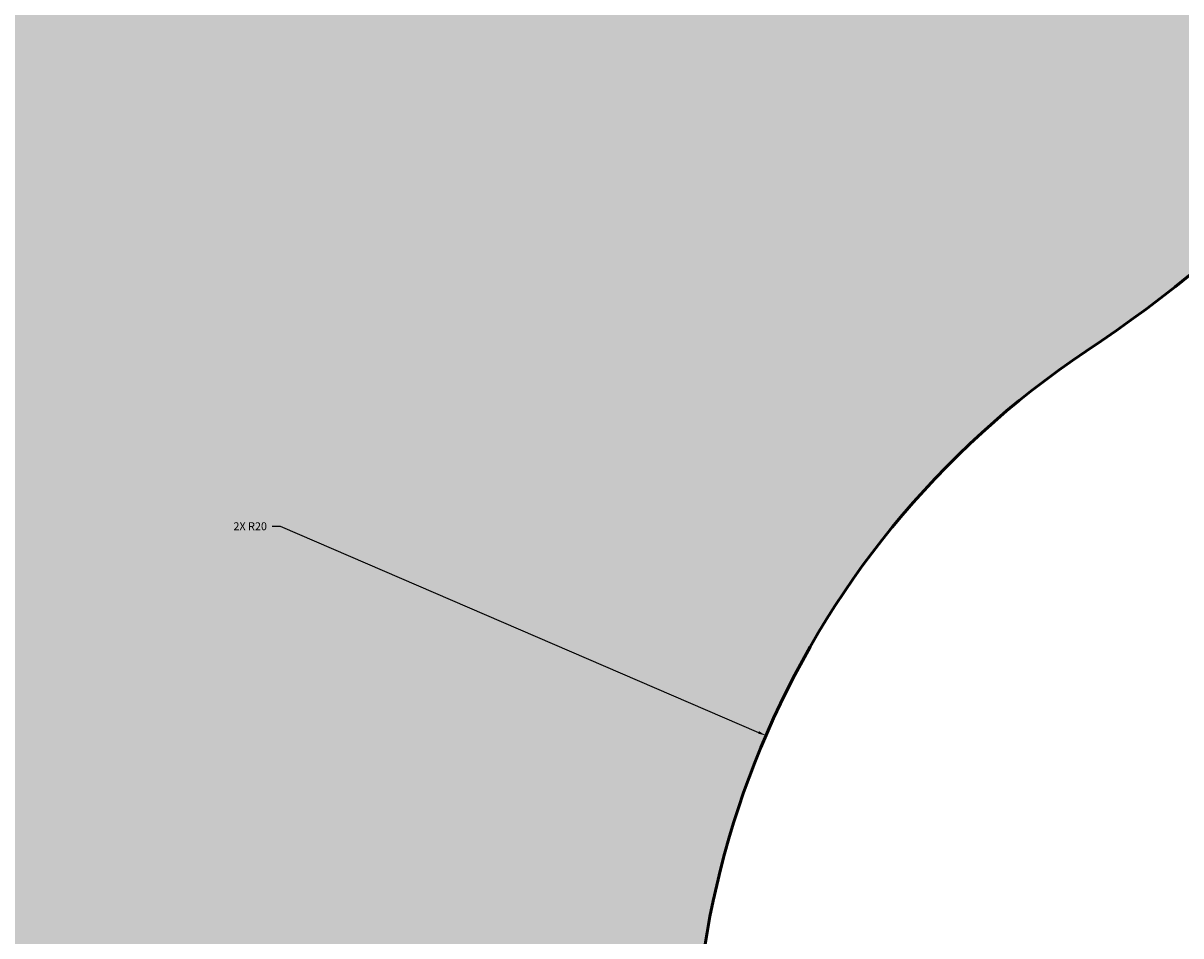
# Model space of a CAD drawing. Units: inches. Extents: x -13 to 107, y -48 to 102.
# Tile 3 of 13: x 22 to 48, y -27 to -7. Entities that reach past the tile are written whole.
import ezdxf

# ---------------------------------------------------------------- set-up
doc = ezdxf.new("R2010")
doc.units = ezdxf.units.IN
doc.header["$MEASUREMENT"] = 0
for name, color, linetype, lineweight in [('M-DIMS', 2, 'Continuous', 18), ('M-HATC', 8, 'Continuous', 18), ('M-OUTL', 7, 'Continuous', 50)]:
    doc.layers.add(name, color=color, linetype=linetype, lineweight=lineweight)
doc.styles.get("Standard").update_dxf_attribs({"font": 'arial.ttf'})
doc.dimstyles.get("Standard").update_dxf_attribs({"dimtxt": 0.18, "dimasz": 0.18, "dimexe": 0.18, "dimexo": 0.0625, "dimgap": 0.09, "dimtad": 0, "dimtih": 1, "dimtoh": 1, "dimdec": 4, "dimzin": 0, "dimdsep": 46, "dimtxsty": 'Standard', "dimcen": 0.09, "dimadec": 0, "dimazin": 0, "dimtfac": 1, "dimtdec": 4, "dimtofl": 0, "dimtmove": 0, "dimatfit": 3, "dimfxl": 1, "dimtolj": 1, "dimtzin": 0, "dimarcsym": 0})

# ---------------------------------------------------------------- blocks, each defined once
blk = doc.blocks.new('*D2')
at = {"layer": 'Defpoints', "color": 0, "transparency": 16777216}
for p in [(-12.585, 94.408), (27.547, 94.408), (27.547, -46.592)]:
    blk.add_point(p, dxfattribs=at)
at = {"layer": 'M-DIMS', "color": 0, "lineweight": -2, "transparency": 16777216}
for p, q in [((27.484, 94.408), (-12.765, 94.408)), ((-12.585, 94.228), (-12.585, 24.088)), ((-12.585, -46.412), (-12.585, 23.727)), ((27.484, -46.592), (-12.765, -46.592))]:
    blk.add_line(p, q, dxfattribs=at)
at = {"layer": 'M-DIMS', "color": 0, "transparency": 16777216}
for points in [[(-12.615, 94.228), (-12.555, 94.228), (-12.585, 94.408)], [(-12.615, -46.412), (-12.555, -46.412), (-12.585, -46.592)]]:
    blk.add_solid(points, dxfattribs=at)
at = {"layer": 'M-DIMS', "color": 0, "transparency": 16777216, "insert": (-12.585, 23.908), "char_height": 0.18, "attachment_point": 5}
blk.add_mtext('\\A1;141', dxfattribs=at)
blk = doc.blocks.new('*D3')
at = {"layer": 'Defpoints', "color": 0, "transparency": 16777216}
for p in [(27.547, 13.408), (67.679, 13.408), (27.547, -36.592)]:
    blk.add_point(p, dxfattribs=at)
at = {"layer": 'M-DIMS', "color": 0, "lineweight": -2, "transparency": 16777216}
for p, q in [((27.609, 13.408), (67.859, 13.408)), ((67.679, 13.228), (67.679, -11.41)), ((67.679, -36.412), (67.679, -11.774)), ((27.609, -36.592), (67.859, -36.592))]:
    blk.add_line(p, q, dxfattribs=at)
at = {"layer": 'M-DIMS', "color": 0, "transparency": 16777216}
for points in [[(67.649, 13.228), (67.709, 13.228), (67.679, 13.408)], [(67.649, -36.412), (67.709, -36.412), (67.679, -36.592)]]:
    blk.add_solid(points, dxfattribs=at)
at = {"layer": 'M-DIMS', "color": 0, "transparency": 16777216, "insert": (67.679, -11.592), "char_height": 0.18, "attachment_point": 5}
blk.add_mtext('\\A1;50', dxfattribs=at)
blk = doc.blocks.new('*D8')
at = {"layer": 'Defpoints', "color": 0, "transparency": 16777216}
for p in [(27.547, 13.408), (50.882, -9.927)]:
    blk.add_point(p, dxfattribs=at)
at = {"layer": 'M-DIMS', "color": 0, "lineweight": -2, "transparency": 16777216}
for p, q in [((27.457, 13.408), (27.637, 13.408)), ((27.547, 13.318), (27.547, 13.498)), ((64.882, -23.927), (51.009, -10.054)), ((65.062, -23.927), (64.882, -23.927))]:
    blk.add_line(p, q, dxfattribs=at)
at = {"layer": 'M-DIMS', "color": 0, "transparency": 16777216}
blk.add_solid([(51.03, -10.033), (50.988, -10.075), (50.882, -9.927)], dxfattribs=at)
at = {"layer": 'M-DIMS', "color": 0, "transparency": 16777216, "insert": (65.562, -23.927), "char_height": 0.18, "attachment_point": 5}
blk.add_mtext('\\A1;2X R33', dxfattribs=at)
blk = doc.blocks.new('*D11')
at = {"layer": 'Defpoints', "color": 0, "transparency": 16777216}
for p in [(38.592, -22.767), (56.959, -30.682)]:
    blk.add_point(p, dxfattribs=at)
at = {"layer": 'M-DIMS', "color": 0, "lineweight": -2, "transparency": 16777216}
for p, q in [((27.392, -18.018), (27.572, -18.018)), ((27.572, -18.018), (38.427, -22.696)), ((56.869, -30.682), (57.049, -30.682)), ((56.959, -30.772), (56.959, -30.592))]:
    blk.add_line(p, q, dxfattribs=at)
at = {"layer": 'M-DIMS', "color": 0, "transparency": 16777216}
blk.add_solid([(38.438, -22.668), (38.415, -22.724), (38.592, -22.767)], dxfattribs=at)
at = {"layer": 'M-DIMS', "color": 0, "transparency": 16777216, "insert": (26.892, -18.018), "char_height": 0.18, "attachment_point": 5}
blk.add_mtext('\\A1;2X R20', dxfattribs=at)

msp = doc.modelspace()

# ---------------------------------------------------------------- hatches: boundary and pattern name
at = {"layer": 'M-HATC'}
h = msp.add_hatch(color=256, dxfattribs=at)
h.set_gradient(color1=(88, 186, 72), color2=(241, 235, 31), tint=1)
h.paths.add_polyline_path([(45.86, -14.044, 0.420873), (54.577, 32.339, -0.184081), (43.437, 76.537, 1.124637), (11.657, 76.537, -0.184081), (0.517, 32.339, 0.420873), (9.234, -14.044, -0.304084), (17.743, -34.622, 1.220926), (37.351, -34.622, -0.304084)])
h.paths.add_polyline_path([(33.479, -5.692, 0.859727), (21.615, -5.692, -0.111692), (13.972, -1.28, 0.859727), (8.04, 8.995, -0.111692), (8.04, 17.82, 0.859727), (13.972, 28.095, -0.111692), (21.615, 32.508, 0.859727), (33.479, 32.508, -0.111692), (41.122, 28.095, 0.859727), (47.054, 17.82, -0.111692), (47.054, 8.995, 0.859727), (41.122, -1.28, -0.111692)], flags=16)
h.paths.add_polyline_path([(32.547, -36.592, -1), (22.547, -36.592, -1)], flags=16)
h.paths.add_polyline_path([(17.547, 78.408, -1), (37.547, 78.408, -1)], flags=16)

# ---------------------------------------------------------------- linework, layer by layer
at = {"layer": 'M-OUTL'}
for centre, radius, start, end in [((27.547, 13.408), 33, 303.707, 35.0067), ((56.959, -30.682), 20, 123.707, 191.3616)]:
    msp.add_arc(centre, radius, start, end, dxfattribs=at)

# ---------------------------------------------------------------- dimensions: what is measured, and where the dimension line sits
at = {"layer": 'M-DIMS'}
for base, p1, p2, picture, middle in [((-12.585, 94.408), (27.547, -46.592), (27.547, 94.408), '*D2', (-12.585, 23.908)), ((67.679, 13.408), (27.547, -36.592), (27.547, 13.408), '*D3', (67.679, -11.592))]:
    dim = msp.add_linear_dim(base=base, p1=p1, p2=p2, angle=90, dimstyle='Standard', override={"dimdec": 0, "dimlfac": 1, "dimrnd": 0, "dimzin": 0, "dimdsep": 46, "dimlunit": 2}, dxfattribs=at)
    dim.commit()
    dim.dimension.update_dxf_attribs({"geometry": picture, "text_midpoint": middle})
for center, mpoint, picture, middle in [((27.547, 13.408), (50.882, -9.927), '*D8', (65.562, -23.927)), ((56.959, -30.682), (38.592, -22.767), '*D11', (26.892, -18.018))]:
    dim = msp.add_radius_dim(center=center, mpoint=mpoint, text='2X <>', dimstyle='Standard', override={"dimdec": 0, "dimlfac": 1, "dimrnd": 0, "dimzin": 0, "dimdsep": 46, "dimlunit": 2}, dxfattribs=at)
    dim.commit()
    dim.dimension.update_dxf_attribs({"geometry": picture, "text_midpoint": middle, "dimtype": 164})

doc.saveas('drawing.dxf')
